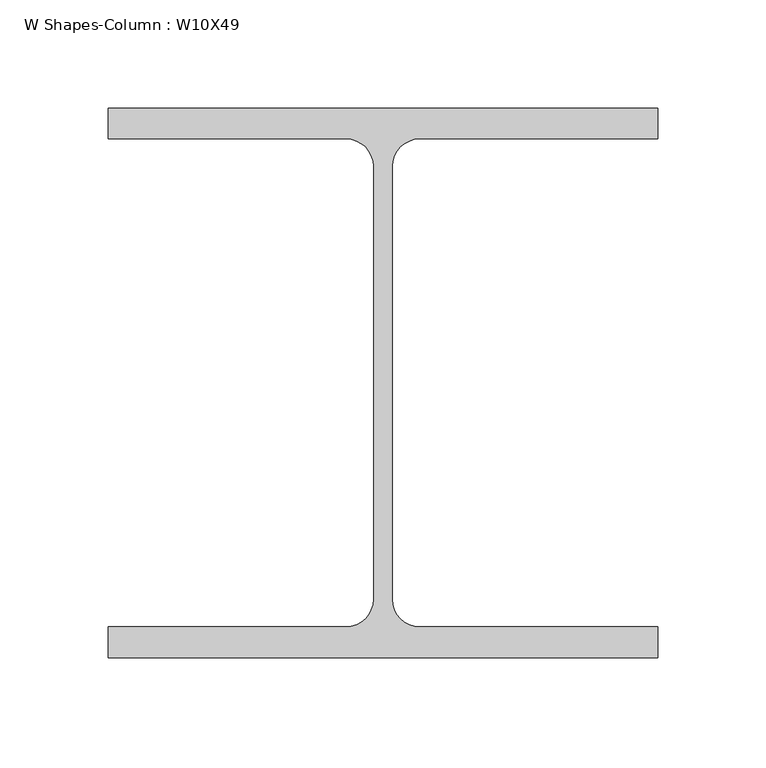
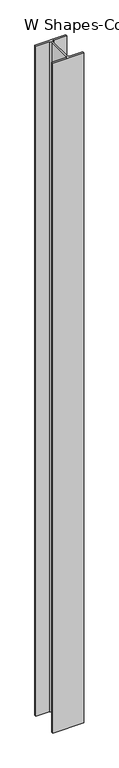
"""IFC4 building model written with IfcOpenShell, lengths in millimetres: column geometry, W Shapes-Column : W10X49."""

from ifc_helpers import new_model, si_unit, point, frame, frame_2d, origin, place, context, project, spatial, polyline, circle_curve, trimmed, segment, composite_curve, outline, extrude, source, transform, mapped, element, save


def w_shapes_column_w10x49_2dae7ecb(model_context):
    return source(origin(), model_context, "Body", "SweptSolid", [
        extrude(outline(composite_curve([segment(polyline([(127.0, 127.0), (127.0, 112.776), (17.018, 112.776)]), True, "CONTINUOUS"), segment(trimmed(circle_curve(frame_2d((17.018, 100.076)), 12.7), [point((17.018, 112.776))], [point((4.318, 100.076))], True, "CARTESIAN"), True, "CONTINUOUS"), segment(polyline([(4.318, 100.076), (4.318, -100.076)]), True, "CONTINUOUS"), segment(trimmed(circle_curve(frame_2d((17.018, -100.076)), 12.7), [point((4.318, -100.076))], [point((17.018, -112.776))], True, "CARTESIAN"), True, "CONTINUOUS"), segment(polyline([(17.018, -112.776), (127.0, -112.776), (127.0, -127.0), (-127.0, -127.0), (-127.0, -112.776), (-17.018, -112.776)]), True, "CONTINUOUS"), segment(trimmed(circle_curve(frame_2d((-17.018, -100.076)), 12.7), [point((-17.018, -112.776))], [point((-4.318, -100.076))], True, "CARTESIAN"), True, "CONTINUOUS"), segment(polyline([(-4.318, -100.076), (-4.318, 100.076)]), True, "CONTINUOUS"), segment(trimmed(circle_curve(frame_2d((-17.018, 100.076)), 12.7), [point((-4.318, 100.076))], [point((-17.018, 112.776))], True, "CARTESIAN"), True, "CONTINUOUS"), segment(polyline([(-17.018, 112.776), (-127.0, 112.776), (-127.0, 127.0), (127.0, 127.0)]), True, "CONTINUOUS")], self_intersect=False)), frame((0.0, 0.0, 304.8), z_axis=(0.0, 0.0, 1.0), x_axis=(1.0, 0.0, 0.0)), (0.0, 0.0, 1.0), 5791.2),
    ])


if __name__ == "__main__":
    model = new_model("IFC4")
    model_context = context("Model", 3, world=origin())
    ifc_project = project(units=[si_unit("LENGTHUNIT", "METRE", prefix="MILLI")], contexts=[model_context])
    site = spatial("IfcSite", under=ifc_project)
    building = spatial("IfcBuilding", under=site)
    placement = place(None, origin())
    w_shapes_column_w10x49_shape = w_shapes_column_w10x49_2dae7ecb(model_context)
    element("IfcColumn", 1, ObjectType="W Shapes-Column : W10X49", at=placement, inside=building, context=model_context, shape_type="MappedRepresentation", body=[
        mapped(w_shapes_column_w10x49_shape, transform((0.0, 0.0, 0.0), x_axis=(1.0, 0.0, 0.0), y_axis=(0.0, 1.0, 0.0), z_axis=(0.0, 0.0, 1.0))),
    ])
    save(model, "model.ifc")

# Revit data of these elements
# Type "W Shapes-Column : W10X49"
#   Section Name Key = "W10x49"
#   Assembly Code = "B10"
#   Width = 10.000"
#   Web Thickness = 0.340"
#   Web Fillet = 0.500"
#   Warping Constant = 2070.00 in⁶
#   Torsional Moment of Inertia = 1.39 in⁴
#   Section Area = 14.40 in²
#   Plastic Modulus weak axis = 28.30 in³
#   Plastic Modulus strong axis = 60.40 in³
#   Perimeter = 58.50 ft²/ft
#   Nominal Weight = 49.00 lbf/ft
#   Moment of Inertia weak axis = 93.40 in⁴
#   Moment of Inertia strong axis = 272.00 in⁴
#   Height = 10.000"
#   Flange Thickness = 0.560"
#   Elastic Modulus weak axis = 18.70 in³
#   Elastic Modulus strong axis = 54.60 in³
#   Centroid Vertical = 5.000"
#   Centroid Horizontal = 5.000"
#   Structural Material [instance default] = Steel ASTM A992
#   Principal Axes Angle = 0
# Element 1 (IfcColumn, "W Shapes-Column : W10X49")
#   Materials on its faces: "Steel ASTM A992"
# Materials
#   "Steel ASTM A992": class "Metal", colour RGB 199 199 199, transparency 0, Description = "Structural steel 50ksi", Cost = 0
